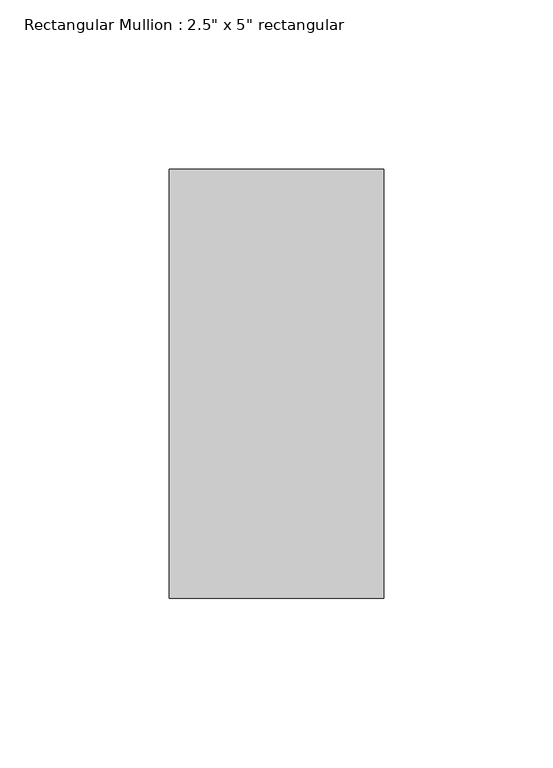
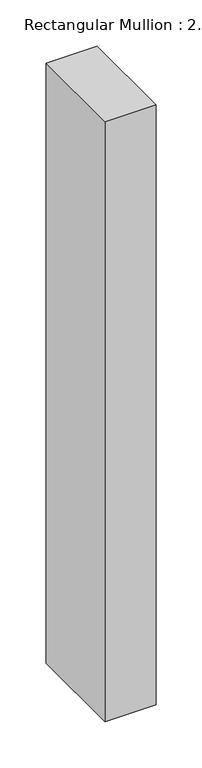
"""IFC4 building model written with IfcOpenShell, lengths in millimetres: member geometry."""

from ifc_helpers import new_model, si_unit, frame, origin, place, context, project, spatial, polyline, outline, extrude, source, transform, mapped, element, save


def member_392009c2(model_context):
    return source(origin(), model_context, "Body", "SweptSolid", [
        extrude(outline(polyline([(0.0, 63.5), (0.0, -63.5), (-63.5, -63.5), (-63.5, 63.5), (0.0, 63.5)])), frame((0.0, 0.0, -791.2941631), z_axis=(0.0, 0.0, 1.0), x_axis=(1.0, 0.0, 0.0)), (0.0, 0.0, 1.0), 791.2941631),
    ])


if __name__ == "__main__":
    model = new_model("IFC4")
    model_context = context("Model", 3, world=origin())
    ifc_project = project(units=[si_unit("LENGTHUNIT", "METRE", prefix="MILLI")], contexts=[model_context])
    site = spatial("IfcSite", under=ifc_project)
    building = spatial("IfcBuilding", under=site)
    placement = place(None, origin())
    member_shape = member_392009c2(model_context)
    element("IfcMember", 1, ObjectType="Rectangular Mullion : 2.5\" x 5\" rectangular", at=placement, inside=building, context=model_context, shape_type="MappedRepresentation", body=[
        mapped(member_shape, transform((0.0, 0.0, 0.0), x_axis=(1.0, 0.0, 0.0), y_axis=(0.0, 1.0, 0.0), z_axis=(0.0, 0.0, 1.0))),
    ])
    save(model, "model.ifc")

# Revit data of these elements
# Type "Rectangular Mullion : 2.5\" x 5\" rectangular"
#   built-in parameter 1007304 = 0.416667 (stored number, unit not read)
#   built-in parameter 1007301 = 0.104167 (stored number, unit not read)
#   built-in parameter 1007300 = 0.104167 (stored number, unit not read)
# Element 1 (IfcMember, "Rectangular Mullion : 2.5\" x 5\" rectangular")
#   Materials on its faces: "Aluminum"
# Materials
#   "Aluminum": class "Metal", colour RGB 247 247 247, transparency 0, Description = "Aluminum 6061", Cost = 0
